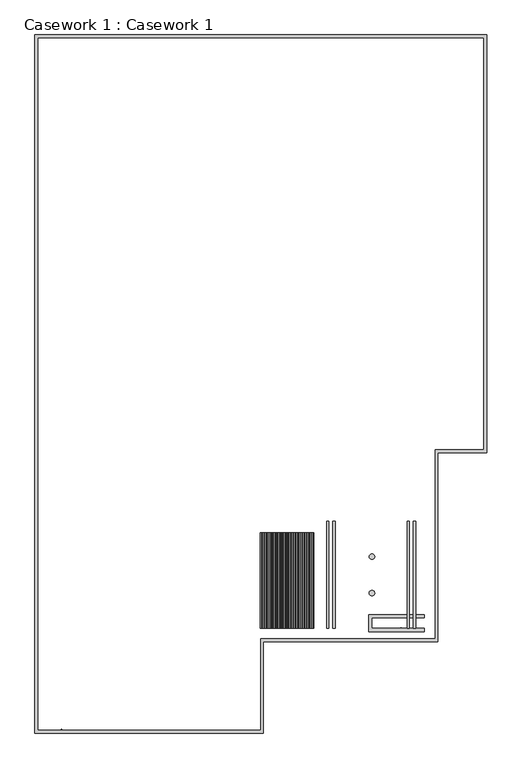
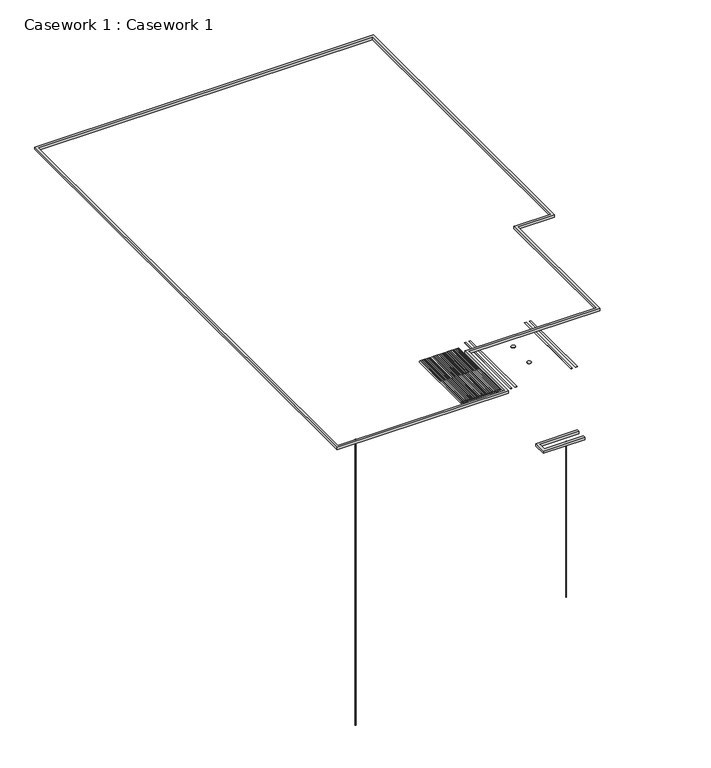
"""IFC4 building model written with IfcOpenShell, lengths in millimetres: furniture geometry, Casework 1 : Casework 1."""

from ifc_helpers import new_model, si_unit, point, frame, frame_2d, origin, origin_with_axes, place, context, project, spatial, polyline, circle_curve, trimmed, segment, composite_curve, outline, extrude, source, transform, mapped, element, save


def casework_1_casework_1_205f5306(model_context):
    return source(origin(), model_context, "Body", "SweptSolid", [
        extrude(outline(polyline([(-283.8712297, -4122.0014262), (-1373.8712297, -4122.0014262), (-1373.8712297, -8352.0014262), (-5273.8712297, -8352.0014262), (-5273.8712297, -10392.0014262), (-10383.8712297, -10392.0014262), (-10383.8712297, 5217.9985738), (-283.8712297, 5217.9985738), (-283.8712297, -4122.0014262)]), holes=[polyline([(-5348.8712297, -10317.0014262), (-5348.8712297, -8277.0014262), (-1448.8712297, -8277.0014262), (-1448.8712297, -4047.0014262), (-358.8712297, -4047.0014262), (-358.8712297, 5142.9985738), (-10308.8712297, 5142.9985738), (-10308.8712297, -10317.0014262), (-5348.8712297, -10317.0014262)])]), frame((0.0, 0.0, 8925.0), z_axis=(0.0, 0.0, 1.0), x_axis=(1.0, 0.0, 0.0)), (0.0, 0.0, 1.0), 75.0),
        extrude(outline(polyline([(-3808.8712297, -8047.0014262), (-3858.8712297, -8047.0014262), (-3858.8712297, -5662.0014262), (-3808.8712297, -5662.0014262), (-3808.8712297, -8047.0014262)])), frame((0.0, 0.0, 7148.0), z_axis=(0.0, 0.0, 1.0), x_axis=(1.0, 0.0, 0.0)), (0.0, 0.0, 1.0), 2.0),
        extrude(outline(polyline([(-3668.8712297, -8047.0014262), (-3718.8712297, -8047.0014262), (-3718.8712297, -5662.0014262), (-3668.8712297, -5662.0014262), (-3668.8712297, -8047.0014262)])), frame((0.0, 0.0, 7148.0), z_axis=(0.0, 0.0, 1.0), x_axis=(1.0, 0.0, 0.0)), (0.0, 0.0, 1.0), 2.0),
        extrude(outline(polyline([(-2008.8712297, -8047.0014262), (-2058.8712297, -8047.0014262), (-2058.8712297, -5662.0014262), (-2008.8712297, -5662.0014262), (-2008.8712297, -8047.0014262)])), frame((0.0, 0.0, 7148.0), z_axis=(0.0, 0.0, 1.0), x_axis=(1.0, 0.0, 0.0)), (0.0, 0.0, 1.0), 2.0),
        extrude(outline(polyline([(-1868.8712297, -8047.0014262), (-1918.8712297, -8047.0014262), (-1918.8712297, -5662.0014262), (-1868.8712297, -5662.0014262), (-1868.8712297, -8047.0014262)])), frame((0.0, 0.0, 7148.0), z_axis=(0.0, 0.0, 1.0), x_axis=(1.0, 0.0, 0.0)), (0.0, 0.0, 1.0), 2.0),
        extrude(outline(composite_curve([segment(trimmed(circle_curve(frame_2d((-2848.8712297, -6446.732503)), 60.0), [point((-2908.8712297, -6446.732503))], [point((-2788.8712297, -6446.732503))], False, "CARTESIAN"), True, "CONTINUOUS"), segment(trimmed(circle_curve(frame_2d((-2848.8712297, -6446.732503)), 60.0), [point((-2788.8712297, -6446.732503))], [point((-2908.8712297, -6446.732503))], False, "CARTESIAN"), True, "CONTINUOUS")], self_intersect=False)), frame((0.0, 0.0, 7148.0), z_axis=(0.0, 0.0, 1.0), x_axis=(1.0, 0.0, 0.0)), (0.0, 0.0, 1.0), 2.0),
        extrude(outline(composite_curve([segment(trimmed(circle_curve(frame_2d((-2848.8712297, -7262.2703493)), 60.0), [point((-2908.8712297, -7262.2703493))], [point((-2788.8712297, -7262.2703493))], False, "CARTESIAN"), True, "CONTINUOUS"), segment(trimmed(circle_curve(frame_2d((-2848.8712297, -7262.2703493)), 60.0), [point((-2788.8712297, -7262.2703493))], [point((-2908.8712297, -7262.2703493))], False, "CARTESIAN"), True, "CONTINUOUS")], self_intersect=False)), frame((0.0, 0.0, 7148.0), z_axis=(0.0, 0.0, 1.0), x_axis=(1.0, 0.0, 0.0)), (0.0, 0.0, 1.0), 2.0),
        extrude(outline(composite_curve([segment(trimmed(circle_curve(frame_2d((7220.4522792, -4171.9999833)), 20.0), [point((7240.4522792, -4171.9999833))], [point((7200.4522792, -4171.9999833))], False, "CARTESIAN"), True, "CONTINUOUS"), segment(trimmed(circle_curve(frame_2d((7220.4522792, -4171.9999833)), 20.0), [point((7200.4522792, -4171.9999833))], [point((7240.4522792, -4171.9999833))], False, "CARTESIAN"), True, "CONTINUOUS")], self_intersect=False)), frame((0.0, -8047.0014262, 0.0), z_axis=(0.0, 1.0, 0.0), x_axis=(0.0, 0.0, 1.0)), (0.0, 0.0, 1.0), 2135.0),
        extrude(outline(composite_curve([segment(trimmed(circle_curve(frame_2d((7220.4522792, -4221.9999833)), 20.0), [point((7240.4522792, -4221.9999833))], [point((7200.4522792, -4221.9999833))], False, "CARTESIAN"), True, "CONTINUOUS"), segment(trimmed(circle_curve(frame_2d((7220.4522792, -4221.9999833)), 20.0), [point((7200.4522792, -4221.9999833))], [point((7240.4522792, -4221.9999833))], False, "CARTESIAN"), True, "CONTINUOUS")], self_intersect=False)), frame((0.0, -8047.0014262, 0.0), z_axis=(0.0, 1.0, 0.0), x_axis=(0.0, 0.0, 1.0)), (0.0, 0.0, 1.0), 2135.0),
        extrude(outline(composite_curve([segment(trimmed(circle_curve(frame_2d((7220.4522792, -4271.9999833)), 20.0), [point((7240.4522792, -4271.9999833))], [point((7200.4522792, -4271.9999833))], False, "CARTESIAN"), True, "CONTINUOUS"), segment(trimmed(circle_curve(frame_2d((7220.4522792, -4271.9999833)), 20.0), [point((7200.4522792, -4271.9999833))], [point((7240.4522792, -4271.9999833))], False, "CARTESIAN"), True, "CONTINUOUS")], self_intersect=False)), frame((0.0, -8047.0014262, 0.0), z_axis=(0.0, 1.0, 0.0), x_axis=(0.0, 0.0, 1.0)), (0.0, 0.0, 1.0), 2135.0),
        extrude(outline(composite_curve([segment(trimmed(circle_curve(frame_2d((7220.4522792, -4321.9999833)), 20.0), [point((7240.4522792, -4321.9999833))], [point((7200.4522792, -4321.9999833))], False, "CARTESIAN"), True, "CONTINUOUS"), segment(trimmed(circle_curve(frame_2d((7220.4522792, -4321.9999833)), 20.0), [point((7200.4522792, -4321.9999833))], [point((7240.4522792, -4321.9999833))], False, "CARTESIAN"), True, "CONTINUOUS")], self_intersect=False)), frame((0.0, -8047.0014262, 0.0), z_axis=(0.0, 1.0, 0.0), x_axis=(0.0, 0.0, 1.0)), (0.0, 0.0, 1.0), 2135.0),
        extrude(outline(composite_curve([segment(trimmed(circle_curve(frame_2d((7220.4522792, -4371.9999833)), 20.0), [point((7240.4522792, -4371.9999833))], [point((7200.4522792, -4371.9999833))], False, "CARTESIAN"), True, "CONTINUOUS"), segment(trimmed(circle_curve(frame_2d((7220.4522792, -4371.9999833)), 20.0), [point((7200.4522792, -4371.9999833))], [point((7240.4522792, -4371.9999833))], False, "CARTESIAN"), True, "CONTINUOUS")], self_intersect=False)), frame((0.0, -8047.0014262, 0.0), z_axis=(0.0, 1.0, 0.0), x_axis=(0.0, 0.0, 1.0)), (0.0, 0.0, 1.0), 2135.0),
        extrude(outline(composite_curve([segment(trimmed(circle_curve(frame_2d((7220.4522792, -4421.9999833)), 20.0), [point((7240.4522792, -4421.9999833))], [point((7200.4522792, -4421.9999833))], False, "CARTESIAN"), True, "CONTINUOUS"), segment(trimmed(circle_curve(frame_2d((7220.4522792, -4421.9999833)), 20.0), [point((7200.4522792, -4421.9999833))], [point((7240.4522792, -4421.9999833))], False, "CARTESIAN"), True, "CONTINUOUS")], self_intersect=False)), frame((0.0, -8047.0014262, 0.0), z_axis=(0.0, 1.0, 0.0), x_axis=(0.0, 0.0, 1.0)), (0.0, 0.0, 1.0), 2135.0),
        extrude(outline(composite_curve([segment(trimmed(circle_curve(frame_2d((7220.4522792, -4471.9999833)), 20.0), [point((7240.4522792, -4471.9999833))], [point((7200.4522792, -4471.9999833))], False, "CARTESIAN"), True, "CONTINUOUS"), segment(trimmed(circle_curve(frame_2d((7220.4522792, -4471.9999833)), 20.0), [point((7200.4522792, -4471.9999833))], [point((7240.4522792, -4471.9999833))], False, "CARTESIAN"), True, "CONTINUOUS")], self_intersect=False)), frame((0.0, -8047.0014262, 0.0), z_axis=(0.0, 1.0, 0.0), x_axis=(0.0, 0.0, 1.0)), (0.0, 0.0, 1.0), 2135.0),
        extrude(outline(composite_curve([segment(trimmed(circle_curve(frame_2d((7220.4522792, -4521.9999833)), 20.0), [point((7240.4522792, -4521.9999833))], [point((7200.4522792, -4521.9999833))], False, "CARTESIAN"), True, "CONTINUOUS"), segment(trimmed(circle_curve(frame_2d((7220.4522792, -4521.9999833)), 20.0), [point((7200.4522792, -4521.9999833))], [point((7240.4522792, -4521.9999833))], False, "CARTESIAN"), True, "CONTINUOUS")], self_intersect=False)), frame((0.0, -8047.0014262, 0.0), z_axis=(0.0, 1.0, 0.0), x_axis=(0.0, 0.0, 1.0)), (0.0, 0.0, 1.0), 2135.0),
        extrude(outline(composite_curve([segment(trimmed(circle_curve(frame_2d((7220.4522792, -4571.9999833)), 20.0), [point((7240.4522792, -4571.9999833))], [point((7200.4522792, -4571.9999833))], False, "CARTESIAN"), True, "CONTINUOUS"), segment(trimmed(circle_curve(frame_2d((7220.4522792, -4571.9999833)), 20.0), [point((7200.4522792, -4571.9999833))], [point((7240.4522792, -4571.9999833))], False, "CARTESIAN"), True, "CONTINUOUS")], self_intersect=False)), frame((0.0, -8047.0014262, 0.0), z_axis=(0.0, 1.0, 0.0), x_axis=(0.0, 0.0, 1.0)), (0.0, 0.0, 1.0), 2135.0),
        extrude(outline(composite_curve([segment(trimmed(circle_curve(frame_2d((7220.4522792, -4621.9999833)), 20.0), [point((7240.4522792, -4621.9999833))], [point((7200.4522792, -4621.9999833))], False, "CARTESIAN"), True, "CONTINUOUS"), segment(trimmed(circle_curve(frame_2d((7220.4522792, -4621.9999833)), 20.0), [point((7200.4522792, -4621.9999833))], [point((7240.4522792, -4621.9999833))], False, "CARTESIAN"), True, "CONTINUOUS")], self_intersect=False)), frame((0.0, -8047.0014262, 0.0), z_axis=(0.0, 1.0, 0.0), x_axis=(0.0, 0.0, 1.0)), (0.0, 0.0, 1.0), 2135.0),
        extrude(outline(composite_curve([segment(trimmed(circle_curve(frame_2d((7220.4522792, -4671.9999833)), 20.0), [point((7240.4522792, -4671.9999833))], [point((7200.4522792, -4671.9999833))], False, "CARTESIAN"), True, "CONTINUOUS"), segment(trimmed(circle_curve(frame_2d((7220.4522792, -4671.9999833)), 20.0), [point((7200.4522792, -4671.9999833))], [point((7240.4522792, -4671.9999833))], False, "CARTESIAN"), True, "CONTINUOUS")], self_intersect=False)), frame((0.0, -8047.0014262, 0.0), z_axis=(0.0, 1.0, 0.0), x_axis=(0.0, 0.0, 1.0)), (0.0, 0.0, 1.0), 2135.0),
        extrude(outline(composite_curve([segment(trimmed(circle_curve(frame_2d((7220.4522792, -4721.9999833)), 20.0), [point((7240.4522792, -4721.9999833))], [point((7200.4522792, -4721.9999833))], False, "CARTESIAN"), True, "CONTINUOUS"), segment(trimmed(circle_curve(frame_2d((7220.4522792, -4721.9999833)), 20.0), [point((7200.4522792, -4721.9999833))], [point((7240.4522792, -4721.9999833))], False, "CARTESIAN"), True, "CONTINUOUS")], self_intersect=False)), frame((0.0, -8047.0014262, 0.0), z_axis=(0.0, 1.0, 0.0), x_axis=(0.0, 0.0, 1.0)), (0.0, 0.0, 1.0), 2135.0),
        extrude(outline(composite_curve([segment(trimmed(circle_curve(frame_2d((7220.4522792, -4771.9999833)), 20.0), [point((7240.4522792, -4771.9999833))], [point((7200.4522792, -4771.9999833))], False, "CARTESIAN"), True, "CONTINUOUS"), segment(trimmed(circle_curve(frame_2d((7220.4522792, -4771.9999833)), 20.0), [point((7200.4522792, -4771.9999833))], [point((7240.4522792, -4771.9999833))], False, "CARTESIAN"), True, "CONTINUOUS")], self_intersect=False)), frame((0.0, -8047.0014262, 0.0), z_axis=(0.0, 1.0, 0.0), x_axis=(0.0, 0.0, 1.0)), (0.0, 0.0, 1.0), 2135.0),
        extrude(outline(composite_curve([segment(trimmed(circle_curve(frame_2d((7220.4522792, -4821.9999833)), 20.0), [point((7240.4522792, -4821.9999833))], [point((7200.4522792, -4821.9999833))], False, "CARTESIAN"), True, "CONTINUOUS"), segment(trimmed(circle_curve(frame_2d((7220.4522792, -4821.9999833)), 20.0), [point((7200.4522792, -4821.9999833))], [point((7240.4522792, -4821.9999833))], False, "CARTESIAN"), True, "CONTINUOUS")], self_intersect=False)), frame((0.0, -8047.0014262, 0.0), z_axis=(0.0, 1.0, 0.0), x_axis=(0.0, 0.0, 1.0)), (0.0, 0.0, 1.0), 2135.0),
        extrude(outline(composite_curve([segment(trimmed(circle_curve(frame_2d((7220.4522792, -4871.9999833)), 20.0), [point((7240.4522792, -4871.9999833))], [point((7200.4522792, -4871.9999833))], False, "CARTESIAN"), True, "CONTINUOUS"), segment(trimmed(circle_curve(frame_2d((7220.4522792, -4871.9999833)), 20.0), [point((7200.4522792, -4871.9999833))], [point((7240.4522792, -4871.9999833))], False, "CARTESIAN"), True, "CONTINUOUS")], self_intersect=False)), frame((0.0, -8047.0014262, 0.0), z_axis=(0.0, 1.0, 0.0), x_axis=(0.0, 0.0, 1.0)), (0.0, 0.0, 1.0), 2135.0),
        extrude(outline(composite_curve([segment(trimmed(circle_curve(frame_2d((7220.4522792, -4921.9999833)), 20.0), [point((7240.4522792, -4921.9999833))], [point((7200.4522792, -4921.9999833))], False, "CARTESIAN"), True, "CONTINUOUS"), segment(trimmed(circle_curve(frame_2d((7220.4522792, -4921.9999833)), 20.0), [point((7200.4522792, -4921.9999833))], [point((7240.4522792, -4921.9999833))], False, "CARTESIAN"), True, "CONTINUOUS")], self_intersect=False)), frame((0.0, -8047.0014262, 0.0), z_axis=(0.0, 1.0, 0.0), x_axis=(0.0, 0.0, 1.0)), (0.0, 0.0, 1.0), 2135.0),
        extrude(outline(composite_curve([segment(trimmed(circle_curve(frame_2d((7220.4522792, -4971.9999833)), 20.0), [point((7240.4522792, -4971.9999833))], [point((7200.4522792, -4971.9999833))], False, "CARTESIAN"), True, "CONTINUOUS"), segment(trimmed(circle_curve(frame_2d((7220.4522792, -4971.9999833)), 20.0), [point((7200.4522792, -4971.9999833))], [point((7240.4522792, -4971.9999833))], False, "CARTESIAN"), True, "CONTINUOUS")], self_intersect=False)), frame((0.0, -8047.0014262, 0.0), z_axis=(0.0, 1.0, 0.0), x_axis=(0.0, 0.0, 1.0)), (0.0, 0.0, 1.0), 2135.0),
        extrude(outline(composite_curve([segment(trimmed(circle_curve(frame_2d((7220.4522792, -5021.9999833)), 20.0), [point((7240.4522792, -5021.9999833))], [point((7200.4522792, -5021.9999833))], False, "CARTESIAN"), True, "CONTINUOUS"), segment(trimmed(circle_curve(frame_2d((7220.4522792, -5021.9999833)), 20.0), [point((7200.4522792, -5021.9999833))], [point((7240.4522792, -5021.9999833))], False, "CARTESIAN"), True, "CONTINUOUS")], self_intersect=False)), frame((0.0, -8047.0014262, 0.0), z_axis=(0.0, 1.0, 0.0), x_axis=(0.0, 0.0, 1.0)), (0.0, 0.0, 1.0), 2135.0),
        extrude(outline(composite_curve([segment(trimmed(circle_curve(frame_2d((7220.4522792, -5071.9999833)), 20.0), [point((7240.4522792, -5071.9999833))], [point((7200.4522792, -5071.9999833))], False, "CARTESIAN"), True, "CONTINUOUS"), segment(trimmed(circle_curve(frame_2d((7220.4522792, -5071.9999833)), 20.0), [point((7200.4522792, -5071.9999833))], [point((7240.4522792, -5071.9999833))], False, "CARTESIAN"), True, "CONTINUOUS")], self_intersect=False)), frame((0.0, -8047.0014262, 0.0), z_axis=(0.0, 1.0, 0.0), x_axis=(0.0, 0.0, 1.0)), (0.0, 0.0, 1.0), 2135.0),
        extrude(outline(composite_curve([segment(trimmed(circle_curve(frame_2d((7220.4522792, -5121.9999833)), 20.0), [point((7240.4522792, -5121.9999833))], [point((7200.4522792, -5121.9999833))], False, "CARTESIAN"), True, "CONTINUOUS"), segment(trimmed(circle_curve(frame_2d((7220.4522792, -5121.9999833)), 20.0), [point((7200.4522792, -5121.9999833))], [point((7240.4522792, -5121.9999833))], False, "CARTESIAN"), True, "CONTINUOUS")], self_intersect=False)), frame((0.0, -8047.0014262, 0.0), z_axis=(0.0, 1.0, 0.0), x_axis=(0.0, 0.0, 1.0)), (0.0, 0.0, 1.0), 2135.0),
        extrude(outline(composite_curve([segment(trimmed(circle_curve(frame_2d((7220.4522792, -5171.9999833)), 20.0), [point((7240.4522792, -5171.9999833))], [point((7200.4522792, -5171.9999833))], False, "CARTESIAN"), True, "CONTINUOUS"), segment(trimmed(circle_curve(frame_2d((7220.4522792, -5171.9999833)), 20.0), [point((7200.4522792, -5171.9999833))], [point((7240.4522792, -5171.9999833))], False, "CARTESIAN"), True, "CONTINUOUS")], self_intersect=False)), frame((0.0, -8047.0014262, 0.0), z_axis=(0.0, 1.0, 0.0), x_axis=(0.0, 0.0, 1.0)), (0.0, 0.0, 1.0), 2135.0),
        extrude(outline(composite_curve([segment(trimmed(circle_curve(frame_2d((7220.4522792, -5221.9999833)), 20.0), [point((7240.4522792, -5221.9999833))], [point((7200.4522792, -5221.9999833))], False, "CARTESIAN"), True, "CONTINUOUS"), segment(trimmed(circle_curve(frame_2d((7220.4522792, -5221.9999833)), 20.0), [point((7200.4522792, -5221.9999833))], [point((7240.4522792, -5221.9999833))], False, "CARTESIAN"), True, "CONTINUOUS")], self_intersect=False)), frame((0.0, -8047.0014262, 0.0), z_axis=(0.0, 1.0, 0.0), x_axis=(0.0, 0.0, 1.0)), (0.0, 0.0, 1.0), 2135.0),
        extrude(outline(composite_curve([segment(trimmed(circle_curve(frame_2d((7220.4522792, -5271.9999833)), 20.0), [point((7240.4522792, -5271.9999833))], [point((7200.4522792, -5271.9999833))], False, "CARTESIAN"), True, "CONTINUOUS"), segment(trimmed(circle_curve(frame_2d((7220.4522792, -5271.9999833)), 20.0), [point((7200.4522792, -5271.9999833))], [point((7240.4522792, -5271.9999833))], False, "CARTESIAN"), True, "CONTINUOUS")], self_intersect=False)), frame((0.0, -8047.0014262, 0.0), z_axis=(0.0, 1.0, 0.0), x_axis=(0.0, 0.0, 1.0)), (0.0, 0.0, 1.0), 2135.0),
        extrude(outline(composite_curve([segment(trimmed(circle_curve(frame_2d((7220.4522792, -5321.9999833)), 20.0), [point((7240.4522792, -5321.9999833))], [point((7200.4522792, -5321.9999833))], False, "CARTESIAN"), True, "CONTINUOUS"), segment(trimmed(circle_curve(frame_2d((7220.4522792, -5321.9999833)), 20.0), [point((7200.4522792, -5321.9999833))], [point((7240.4522792, -5321.9999833))], False, "CARTESIAN"), True, "CONTINUOUS")], self_intersect=False)), frame((0.0, -8047.0014262, 0.0), z_axis=(0.0, 1.0, 0.0), x_axis=(0.0, 0.0, 1.0)), (0.0, 0.0, 1.0), 2135.0),
        extrude(outline(polyline([(-1678.8712297, -8047.0014262), (-1678.8712297, -8122.0014262), (-2923.8712297, -8122.0014262), (-2923.8712297, -7742.0014262), (-1678.8712297, -7742.0014262), (-1678.8712297, -7817.0014262), (-2848.8712297, -7817.0014262), (-2848.8712297, -8047.0014262), (-1678.8712297, -8047.0014262)])), frame((0.0, 0.0, 4825.0), z_axis=(0.0, 0.0, 1.0), x_axis=(1.0, 0.0, 0.0)), (0.0, 0.0, 1.0), 75.0),
        extrude(outline(composite_curve([segment(trimmed(circle_curve(frame_2d((-2198.8712297, -8047.0014262)), 7.5), [point((-2206.3712297, -8047.0014262))], [point((-2191.3712297, -8047.0014262))], False, "CARTESIAN"), True, "CONTINUOUS"), segment(polyline([(-2191.3712297, -8047.0014262), (-2189.8757624, -8047.0014262), (-2189.8757624, -8052.2945745), (-2208.7196944, -8052.2945745), (-2208.7196944, -8047.0014262), (-2206.3712297, -8047.0014262)]), True, "CONTINUOUS")], self_intersect=False)), origin_with_axes(), (0.0, 0.0, 1.0), 4900.0),
        extrude(outline(composite_curve([segment(trimmed(circle_curve(frame_2d((-9788.8712297, -10317.0014262)), 7.5), [point((-9788.8712297, -10309.5014262))], [point((-9781.3712297, -10317.0014262))], False, "CARTESIAN"), True, "CONTINUOUS"), segment(polyline([(-9781.3712297, -10317.0014262), (-9777.7993979, -10317.0014262), (-9777.7993979, -10322.0014262), (-9799.9430614, -10322.0014262), (-9799.9430614, -10317.0014262), (-9796.3712297, -10317.0014262)]), True, "CONTINUOUS"), segment(trimmed(circle_curve(frame_2d((-9788.8712297, -10317.0014262)), 7.5), [point((-9796.3712297, -10317.0014262))], [point((-9788.8712297, -10309.5014262))], False, "CARTESIAN"), True, "CONTINUOUS")], self_intersect=False)), origin_with_axes(), (0.0, 0.0, 1.0), 9000.0),
    ])


if __name__ == "__main__":
    model = new_model("IFC4")
    model_context = context("Model", 3, world=origin())
    ifc_project = project(units=[si_unit("LENGTHUNIT", "METRE", prefix="MILLI")], contexts=[model_context])
    site = spatial("IfcSite", under=ifc_project)
    building = spatial("IfcBuilding", under=site)
    placement = place(None, origin())
    casework_1_casework_1_shape = casework_1_casework_1_205f5306(model_context)
    element("IfcFurniture", 1, ObjectType="Casework 1 : Casework 1", at=placement, inside=building, context=model_context, shape_type="MappedRepresentation", body=[
        mapped(casework_1_casework_1_shape, transform((0.0, 0.0, 0.0), x_axis=(1.0, 0.0, 0.0), y_axis=(0.0, 1.0, 0.0), z_axis=(0.0, 0.0, 1.0))),
    ])
    save(model, "model.ifc")

# Revit data of these elements
# Element 1 (IfcFurniture, "Casework 1 : Casework 1")
#   Materials on its faces: "Iron, Ductile", "J LIGHT", "J POP"
# Materials
#   "Iron, Ductile": class "Metal", colour RGB 90 97 102, transparency 0, Description = "Ductile cast iron", Cost = 0
#   "J LIGHT": class "Generic", colour RGB 255 255 0, transparency 0, Cost = 0
#   "J POP": class "Generic", colour RGB 255 255 255, transparency 0, Cost = 0
